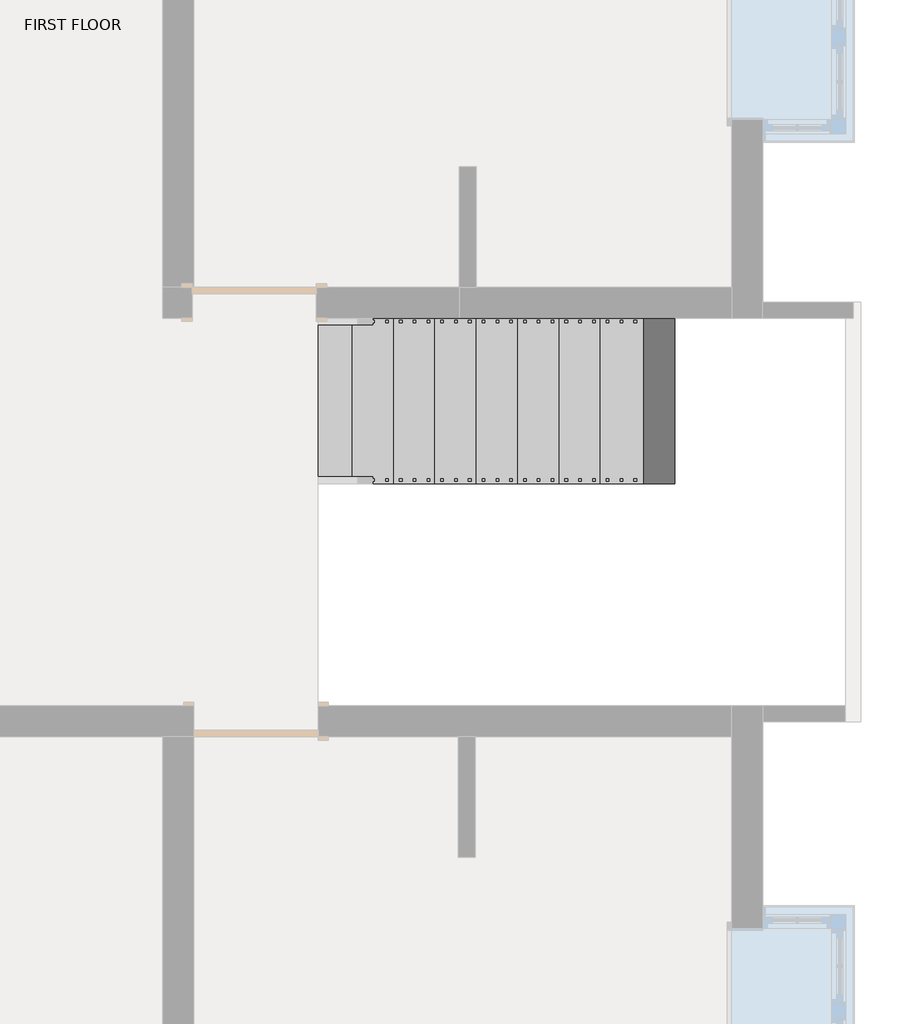
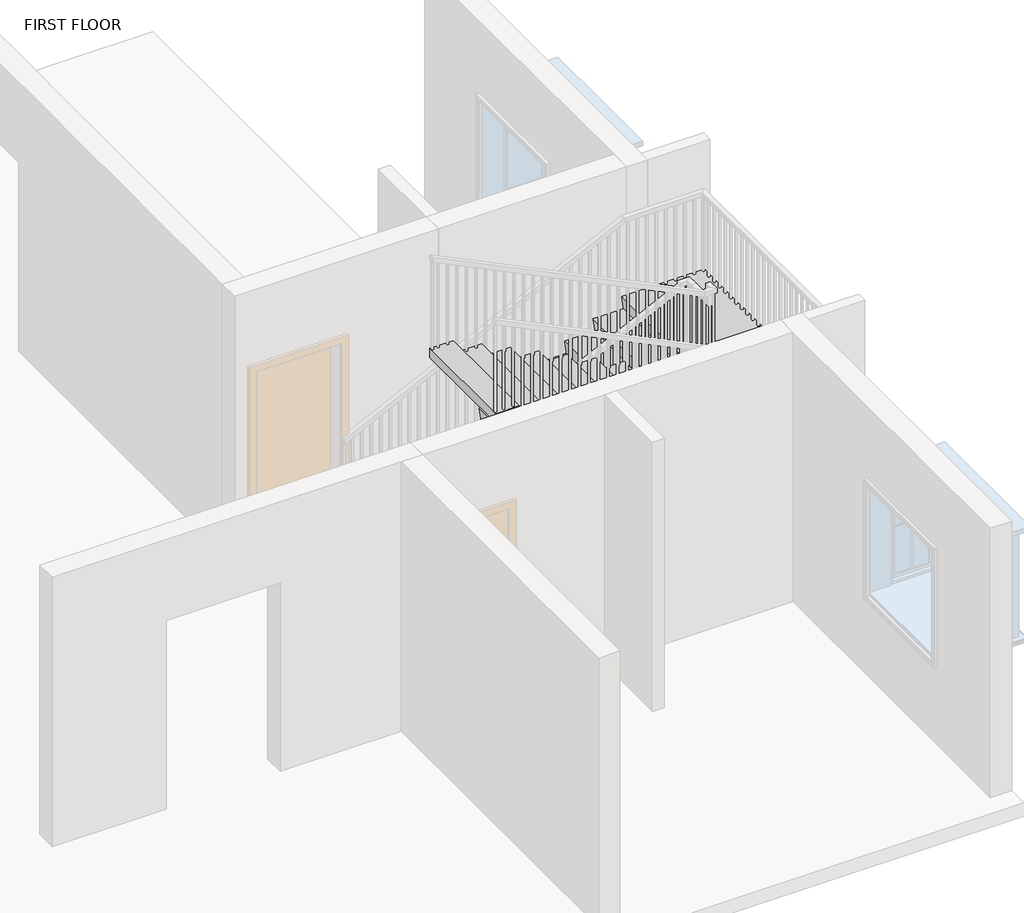
# One storey, part 3 of 6: 1 railing, 1 stair flight.
"""IFC4 building model written with IfcOpenShell, lengths in millimetres."""

from ifc_helpers import new_model, si_unit, frame, origin, place, context, project, spatial, polyline, outline, extrude, faceted_brep, element, save

model = new_model("IFC4")

# Units and contexts
model_context = context("Model", 3, world=origin())
ifc_project = project(units=[si_unit("LENGTHUNIT", "METRE", prefix="MILLI")], contexts=[model_context])

# Site, building, storey
site = spatial("IfcSite", under=ifc_project)
building = spatial("IfcBuilding", under=site)
storey = spatial("IfcBuildingStorey", under=building, Name="FIRST FLOOR", Elevation=3200.4)

# Railing
placement = place(None, origin())
element("IfcRailing", 1, ObjectType="Handrail - Rectangular", at=placement, inside=storey, context=model_context, shape_type="SolidModel", body=[
    faceted_brep([(3126.2584916, -947.666654, 4260.2727273), (3126.2584916, -947.666654, 4203.7956113), (3126.2584916, -998.466654, 4203.7956113), (3126.2584916, -998.466654, 4260.2727273), (6044.5829507, -947.666654, 5677.9823634), (6095.3829507, -947.666654, 5646.1836718), (6095.3829507, -998.466654, 5646.1836718), (6044.5829507, -998.466654, 5677.9823634), (6044.5829507, -947.666654, 5715.0), (6095.3829507, -947.666654, 5664.2), (6095.3829507, -998.466654, 5664.2), (6044.5829507, -998.466654, 5715.0), (6171.5829507, -947.666654, 5715.0), (6171.5829507, -947.666654, 5664.2), (6120.7829507, -998.466654, 5664.2), (6120.7829507, -998.466654, 5715.0), (6171.5829507, -1074.666654, 5715.0), (6171.5829507, -1074.666654, 5664.2), (6120.7829507, -1074.666654, 5664.2), (6120.7829507, -1074.666654, 5715.0), (6171.5829507, -1341.366654, 5715.0), (6171.5829507, -1392.166654, 5664.2), (6120.7829507, -1392.166654, 5664.2), (6120.7829507, -1341.366654, 5715.0), (6171.5829507, -1341.366654, 5897.4903639), (6171.5829507, -1392.166654, 5846.6903639), (6120.7829507, -1392.166654, 5846.6903639), (6120.7829507, -1341.366654, 5897.4903639), (6171.5829507, -1468.366654, 5897.4903639), (6171.5829507, -1468.366654, 5846.6903639), (6120.7829507, -1417.566654, 5846.6903639), (6120.7829507, -1417.566654, 5897.4903639), (6044.5829507, -1468.366654, 5897.4903639), (6032.8967309, -1468.366654, 5846.6903639), (6032.8967309, -1417.566654, 5846.6903639), (6044.5829507, -1417.566654, 5897.4903639), (3126.2584916, -1468.366654, 7315.2), (3126.2584916, -1417.566654, 7315.2), (3126.2584916, -1417.566654, 7258.722884), (3126.2584916, -1468.366654, 7258.722884)], [[[0, 1, 2, 3]], [[1, 0, 4, 5]], [[2, 1, 5, 6]], [[3, 2, 6, 7]], [[0, 3, 7, 4]], [[5, 4, 8, 9]], [[6, 5, 9, 10]], [[7, 6, 10, 11]], [[4, 7, 11, 8]], [[9, 8, 12, 13]], [[10, 9, 13, 14]], [[11, 10, 14, 15]], [[8, 11, 15, 12]], [[13, 12, 16, 17]], [[14, 13, 17, 18]], [[15, 14, 18, 19]], [[12, 15, 19, 16]], [[17, 16, 20, 21]], [[18, 17, 21, 22]], [[19, 18, 22, 23]], [[16, 19, 23, 20]], [[21, 20, 24, 25]], [[22, 21, 25, 26]], [[23, 22, 26, 27]], [[20, 23, 27, 24]], [[25, 24, 28, 29]], [[26, 25, 29, 30]], [[27, 26, 30, 31]], [[24, 27, 31, 28]], [[29, 28, 32, 33]], [[30, 29, 33, 34]], [[31, 30, 34, 35]], [[28, 31, 35, 32]], [[36, 37, 38, 39]], [[33, 32, 36, 39]], [[34, 33, 39, 38]], [[35, 34, 38, 37]], [[32, 35, 37, 36]]]),
    extrude(outline(polyline([(7218.3778093, 3209.3079507), (7227.6322184, 3190.2579507), (6255.3272727, 3190.2579507), (6255.3272727, 3209.3079507), (7218.3778093, 3209.3079507)])), frame((0.0, -1452.491654, 0.0), z_axis=(0.0, 1.0, 0.0), x_axis=(0.0, 0.0, 1.0)), (0.0, 0.0, 1.0), 19.05),
    extrude(outline(polyline([(7169.0209605, 3310.9079507), (7178.2753696, 3291.8579507), (6255.3272727, 3291.8579507), (6255.3272727, 3310.9079507), (7169.0209605, 3310.9079507)])), frame((0.0, -1452.491654, 0.0), z_axis=(0.0, 1.0, 0.0), x_axis=(0.0, 0.0, 1.0)), (0.0, 0.0, 1.0), 19.05),
    extrude(outline(polyline([(7119.6641117, 3412.5079507), (7128.9185208, 3393.4579507), (6109.8545455, 3393.4579507), (6109.8545455, 3412.5079507), (7119.6641117, 3412.5079507)])), frame((0.0, -1452.491654, 0.0), z_axis=(0.0, 1.0, 0.0), x_axis=(0.0, 0.0, 1.0)), (0.0, 0.0, 1.0), 19.05),
    extrude(outline(polyline([(7070.3072629, 3514.1079507), (7079.5616721, 3495.0579507), (6109.8545455, 3495.0579507), (6109.8545455, 3514.1079507), (7070.3072629, 3514.1079507)])), frame((0.0, -1452.491654, 0.0), z_axis=(0.0, 1.0, 0.0), x_axis=(0.0, 0.0, 1.0)), (0.0, 0.0, 1.0), 19.05),
    extrude(outline(polyline([(7020.9504141, 3615.7079507), (7030.2048233, 3596.6579507), (6109.8545455, 3596.6579507), (6109.8545455, 3615.7079507), (7020.9504141, 3615.7079507)])), frame((0.0, -1452.491654, 0.0), z_axis=(0.0, 1.0, 0.0), x_axis=(0.0, 0.0, 1.0)), (0.0, 0.0, 1.0), 19.05),
    extrude(outline(polyline([(6971.5935653, 3717.3079507), (6980.8479745, 3698.2579507), (5964.3818182, 3698.2579507), (5964.3818182, 3717.3079507), (6971.5935653, 3717.3079507)])), frame((0.0, -1452.491654, 0.0), z_axis=(0.0, 1.0, 0.0), x_axis=(0.0, 0.0, 1.0)), (0.0, 0.0, 1.0), 19.05),
    extrude(outline(polyline([(6922.2367166, 3818.9079507), (6931.4911257, 3799.8579507), (5964.3818182, 3799.8579507), (5964.3818182, 3818.9079507), (6922.2367166, 3818.9079507)])), frame((0.0, -1452.491654, 0.0), z_axis=(0.0, 1.0, 0.0), x_axis=(0.0, 0.0, 1.0)), (0.0, 0.0, 1.0), 19.05),
    extrude(outline(polyline([(6872.8798678, 3920.5079507), (6882.1342769, 3901.4579507), (5964.3818182, 3901.4579507), (5964.3818182, 3920.5079507), (6872.8798678, 3920.5079507)])), frame((0.0, -1452.491654, 0.0), z_axis=(0.0, 1.0, 0.0), x_axis=(0.0, 0.0, 1.0)), (0.0, 0.0, 1.0), 19.05),
    extrude(outline(polyline([(6823.523019, 4022.1079507), (6832.7774281, 4003.0579507), (5818.9090909, 4003.0579507), (5818.9090909, 4022.1079507), (6823.523019, 4022.1079507)])), frame((0.0, -1452.491654, 0.0), z_axis=(0.0, 1.0, 0.0), x_axis=(0.0, 0.0, 1.0)), (0.0, 0.0, 1.0), 19.05),
    extrude(outline(polyline([(6774.1661702, 4123.7079507), (6783.4205793, 4104.6579507), (5818.9090909, 4104.6579507), (5818.9090909, 4123.7079507), (6774.1661702, 4123.7079507)])), frame((0.0, -1452.491654, 0.0), z_axis=(0.0, 1.0, 0.0), x_axis=(0.0, 0.0, 1.0)), (0.0, 0.0, 1.0), 19.05),
    extrude(outline(polyline([(6724.8093214, 4225.3079507), (6734.0637306, 4206.2579507), (5818.9090909, 4206.2579507), (5818.9090909, 4225.3079507), (6724.8093214, 4225.3079507)])), frame((0.0, -1452.491654, 0.0), z_axis=(0.0, 1.0, 0.0), x_axis=(0.0, 0.0, 1.0)), (0.0, 0.0, 1.0), 19.05),
    extrude(outline(polyline([(6675.4524726, 4326.9079507), (6684.7068818, 4307.8579507), (5673.4363636, 4307.8579507), (5673.4363636, 4326.9079507), (6675.4524726, 4326.9079507)])), frame((0.0, -1452.491654, 0.0), z_axis=(0.0, 1.0, 0.0), x_axis=(0.0, 0.0, 1.0)), (0.0, 0.0, 1.0), 19.05),
    extrude(outline(polyline([(6626.0956238, 4428.5079507), (6635.350033, 4409.4579507), (5673.4363636, 4409.4579507), (5673.4363636, 4428.5079507), (6626.0956238, 4428.5079507)])), frame((0.0, -1452.491654, 0.0), z_axis=(0.0, 1.0, 0.0), x_axis=(0.0, 0.0, 1.0)), (0.0, 0.0, 1.0), 19.05),
    extrude(outline(polyline([(6576.7387751, 4530.1079507), (6585.9931842, 4511.0579507), (5673.4363636, 4511.0579507), (5673.4363636, 4530.1079507), (6576.7387751, 4530.1079507)])), frame((0.0, -1452.491654, 0.0), z_axis=(0.0, 1.0, 0.0), x_axis=(0.0, 0.0, 1.0)), (0.0, 0.0, 1.0), 19.05),
    extrude(outline(polyline([(6527.3819263, 4631.7079507), (6536.6363354, 4612.6579507), (5527.9636364, 4612.6579507), (5527.9636364, 4631.7079507), (6527.3819263, 4631.7079507)])), frame((0.0, -1452.491654, 0.0), z_axis=(0.0, 1.0, 0.0), x_axis=(0.0, 0.0, 1.0)), (0.0, 0.0, 1.0), 19.05),
    extrude(outline(polyline([(6478.0250775, 4733.3079507), (6487.2794866, 4714.2579507), (5527.9636364, 4714.2579507), (5527.9636364, 4733.3079507), (6478.0250775, 4733.3079507)])), frame((0.0, -1452.491654, 0.0), z_axis=(0.0, 1.0, 0.0), x_axis=(0.0, 0.0, 1.0)), (0.0, 0.0, 1.0), 19.05),
    extrude(outline(polyline([(6428.6682287, 4834.9079507), (6437.9226379, 4815.8579507), (5527.9636364, 4815.8579507), (5527.9636364, 4834.9079507), (6428.6682287, 4834.9079507)])), frame((0.0, -1452.491654, 0.0), z_axis=(0.0, 1.0, 0.0), x_axis=(0.0, 0.0, 1.0)), (0.0, 0.0, 1.0), 19.05),
    extrude(outline(polyline([(6379.3113799, 4936.5079507), (6388.5657891, 4917.4579507), (5382.4909091, 4917.4579507), (5382.4909091, 4936.5079507), (6379.3113799, 4936.5079507)])), frame((0.0, -1452.491654, 0.0), z_axis=(0.0, 1.0, 0.0), x_axis=(0.0, 0.0, 1.0)), (0.0, 0.0, 1.0), 19.05),
    extrude(outline(polyline([(6329.9545311, 5038.1079507), (6339.2089403, 5019.0579507), (5382.4909091, 5019.0579507), (5382.4909091, 5038.1079507), (6329.9545311, 5038.1079507)])), frame((0.0, -1452.491654, 0.0), z_axis=(0.0, 1.0, 0.0), x_axis=(0.0, 0.0, 1.0)), (0.0, 0.0, 1.0), 19.05),
    extrude(outline(polyline([(6280.5976824, 5139.7079507), (6289.8520915, 5120.6579507), (5382.4909091, 5120.6579507), (5382.4909091, 5139.7079507), (6280.5976824, 5139.7079507)])), frame((0.0, -1452.491654, 0.0), z_axis=(0.0, 1.0, 0.0), x_axis=(0.0, 0.0, 1.0)), (0.0, 0.0, 1.0), 19.05),
    extrude(outline(polyline([(6231.159384, 5241.3079507), (6240.4137931, 5222.2579507), (5237.0181818, 5222.2579507), (5237.0181818, 5241.3079507), (6231.159384, 5241.3079507)])), frame((0.0, -1452.491654, 0.0), z_axis=(0.0, 1.0, 0.0), x_axis=(0.0, 0.0, 1.0)), (0.0, 0.0, 1.0), 19.05),
    extrude(outline(polyline([(6181.8839848, 5342.9079507), (6191.1383939, 5323.8579507), (5237.0181818, 5323.8579507), (5237.0181818, 5342.9079507), (6181.8839848, 5342.9079507)])), frame((0.0, -1452.491654, 0.0), z_axis=(0.0, 1.0, 0.0), x_axis=(0.0, 0.0, 1.0)), (0.0, 0.0, 1.0), 19.05),
    extrude(outline(polyline([(6132.527136, 5444.5079507), (6141.7815452, 5425.4579507), (5237.0181818, 5425.4579507), (5237.0181818, 5444.5079507), (6132.527136, 5444.5079507)])), frame((0.0, -1452.491654, 0.0), z_axis=(0.0, 1.0, 0.0), x_axis=(0.0, 0.0, 1.0)), (0.0, 0.0, 1.0), 19.05),
    extrude(outline(polyline([(6083.1702872, 5546.1079507), (6092.4246964, 5527.0579507), (5091.5454545, 5527.0579507), (5091.5454545, 5546.1079507), (6083.1702872, 5546.1079507)])), frame((0.0, -1452.491654, 0.0), z_axis=(0.0, 1.0, 0.0), x_axis=(0.0, 0.0, 1.0)), (0.0, 0.0, 1.0), 19.05),
    extrude(outline(polyline([(6033.8134384, 5647.7079507), (6043.0678476, 5628.6579507), (5091.5454545, 5628.6579507), (5091.5454545, 5647.7079507), (6033.8134384, 5647.7079507)])), frame((0.0, -1452.491654, 0.0), z_axis=(0.0, 1.0, 0.0), x_axis=(0.0, 0.0, 1.0)), (0.0, 0.0, 1.0), 19.05),
    extrude(outline(polyline([(5984.4565897, 5749.3079507), (5993.7109988, 5730.2579507), (5091.5454545, 5730.2579507), (5091.5454545, 5749.3079507), (5984.4565897, 5749.3079507)])), frame((0.0, -1452.491654, 0.0), z_axis=(0.0, 1.0, 0.0), x_axis=(0.0, 0.0, 1.0)), (0.0, 0.0, 1.0), 19.05),
    extrude(outline(polyline([(5935.0997409, 5850.9079507), (5944.35415, 5831.8579507), (4946.0727273, 5831.8579507), (4946.0727273, 5850.9079507), (5935.0997409, 5850.9079507)])), frame((0.0, -1452.491654, 0.0), z_axis=(0.0, 1.0, 0.0), x_axis=(0.0, 0.0, 1.0)), (0.0, 0.0, 1.0), 19.05),
    extrude(outline(polyline([(5885.7428921, 5952.5079507), (5894.9973012, 5933.4579507), (4946.0727273, 5933.4579507), (4946.0727273, 5952.5079507), (5885.7428921, 5952.5079507)])), frame((0.0, -1452.491654, 0.0), z_axis=(0.0, 1.0, 0.0), x_axis=(0.0, 0.0, 1.0)), (0.0, 0.0, 1.0), 19.05),
    extrude(outline(polyline([(5836.3860433, 6054.1079507), (5845.6404524, 6035.0579507), (4946.0727273, 6035.0579507), (4946.0727273, 6054.1079507), (5836.3860433, 6054.1079507)])), frame((0.0, -1452.491654, 0.0), z_axis=(0.0, 1.0, 0.0), x_axis=(0.0, 0.0, 1.0)), (0.0, 0.0, 1.0), 19.05),
    extrude(outline(polyline([(6136.6579507, -1369.941654), (6155.7079507, -1369.941654), (6155.7079507, -1388.991654), (6136.6579507, -1388.991654), (6136.6579507, -1369.941654)])), frame((0.0, 0.0, 4800.6), z_axis=(0.0, 0.0, 1.0), x_axis=(1.0, 0.0, 0.0)), (0.0, 0.0, 1.0), 1046.0903639),
    extrude(outline(polyline([(6136.6579507, -1268.341654), (6155.7079507, -1268.341654), (6155.7079507, -1287.391654), (6136.6579507, -1287.391654), (6136.6579507, -1268.341654)])), frame((0.0, 0.0, 4800.6), z_axis=(0.0, 0.0, 1.0), x_axis=(1.0, 0.0, 0.0)), (0.0, 0.0, 1.0), 863.6),
    extrude(outline(polyline([(6136.6579507, -1166.741654), (6155.7079507, -1166.741654), (6155.7079507, -1185.791654), (6136.6579507, -1185.791654), (6136.6579507, -1166.741654)])), frame((0.0, 0.0, 4800.6), z_axis=(0.0, 0.0, 1.0), x_axis=(1.0, 0.0, 0.0)), (0.0, 0.0, 1.0), 863.6),
    extrude(outline(polyline([(6136.6579507, -1065.141654), (6155.7079507, -1065.141654), (6155.7079507, -1084.191654), (6136.6579507, -1084.191654), (6136.6579507, -1065.141654)])), frame((0.0, 0.0, 4800.6), z_axis=(0.0, 0.0, 1.0), x_axis=(1.0, 0.0, 0.0)), (0.0, 0.0, 1.0), 863.6),
    extrude(outline(polyline([(6063.1334916, -982.591654), (6063.1334916, -963.541654), (6082.1834916, -963.541654), (6082.1834916, -982.591654), (6063.1334916, -982.591654)])), frame((0.0, 0.0, 4655.1272727), z_axis=(0.0, 0.0, 1.0), x_axis=(1.0, 0.0, 0.0)), (0.0, 0.0, 1.0), 1009.0727273),
    extrude(outline(polyline([(5590.4145818, 5980.5834916), (5581.1601727, 5961.5334916), (4655.1272727, 5961.5334916), (4655.1272727, 5980.5834916), (5590.4145818, 5980.5834916)])), frame((0.0, -982.591654, 0.0), z_axis=(0.0, 1.0, 0.0), x_axis=(0.0, 0.0, 1.0)), (0.0, 0.0, 1.0), 19.05),
    extrude(outline(polyline([(5541.057733, 5878.9834916), (5531.8033239, 5859.9334916), (4655.1272727, 5859.9334916), (4655.1272727, 5878.9834916), (5541.057733, 5878.9834916)])), frame((0.0, -982.591654, 0.0), z_axis=(0.0, 1.0, 0.0), x_axis=(0.0, 0.0, 1.0)), (0.0, 0.0, 1.0), 19.05),
    extrude(outline(polyline([(5491.7008843, 5777.3834916), (5482.4464751, 5758.3334916), (4509.6545455, 5758.3334916), (4509.6545455, 5777.3834916), (5491.7008843, 5777.3834916)])), frame((0.0, -982.591654, 0.0), z_axis=(0.0, 1.0, 0.0), x_axis=(0.0, 0.0, 1.0)), (0.0, 0.0, 1.0), 19.05),
    extrude(outline(polyline([(5442.3440355, 5675.7834916), (5433.0896263, 5656.7334916), (4509.6545455, 5656.7334916), (4509.6545455, 5675.7834916), (5442.3440355, 5675.7834916)])), frame((0.0, -982.591654, 0.0), z_axis=(0.0, 1.0, 0.0), x_axis=(0.0, 0.0, 1.0)), (0.0, 0.0, 1.0), 19.05),
    extrude(outline(polyline([(5392.9871867, 5574.1834916), (5383.7327775, 5555.1334916), (4509.6545455, 5555.1334916), (4509.6545455, 5574.1834916), (5392.9871867, 5574.1834916)])), frame((0.0, -982.591654, 0.0), z_axis=(0.0, 1.0, 0.0), x_axis=(0.0, 0.0, 1.0)), (0.0, 0.0, 1.0), 19.05),
    extrude(outline(polyline([(5343.6303379, 5472.5834916), (5334.3759288, 5453.5334916), (4364.1818182, 5453.5334916), (4364.1818182, 5472.5834916), (5343.6303379, 5472.5834916)])), frame((0.0, -982.591654, 0.0), z_axis=(0.0, 1.0, 0.0), x_axis=(0.0, 0.0, 1.0)), (0.0, 0.0, 1.0), 19.05),
    extrude(outline(polyline([(5294.2734891, 5370.9834916), (5285.01908, 5351.9334916), (4364.1818182, 5351.9334916), (4364.1818182, 5370.9834916), (5294.2734891, 5370.9834916)])), frame((0.0, -982.591654, 0.0), z_axis=(0.0, 1.0, 0.0), x_axis=(0.0, 0.0, 1.0)), (0.0, 0.0, 1.0), 19.05),
    extrude(outline(polyline([(5244.9166403, 5269.3834916), (5235.6622312, 5250.3334916), (4364.1818182, 5250.3334916), (4364.1818182, 5269.3834916), (5244.9166403, 5269.3834916)])), frame((0.0, -982.591654, 0.0), z_axis=(0.0, 1.0, 0.0), x_axis=(0.0, 0.0, 1.0)), (0.0, 0.0, 1.0), 19.05),
    extrude(outline(polyline([(5195.5597915, 5167.7834916), (5186.3053824, 5148.7334916), (4218.7090909, 5148.7334916), (4218.7090909, 5167.7834916), (5195.5597915, 5167.7834916)])), frame((0.0, -982.591654, 0.0), z_axis=(0.0, 1.0, 0.0), x_axis=(0.0, 0.0, 1.0)), (0.0, 0.0, 1.0), 19.05),
    extrude(outline(polyline([(5146.2029428, 5066.1834916), (5136.9485336, 5047.1334916), (4218.7090909, 5047.1334916), (4218.7090909, 5066.1834916), (5146.2029428, 5066.1834916)])), frame((0.0, -982.591654, 0.0), z_axis=(0.0, 1.0, 0.0), x_axis=(0.0, 0.0, 1.0)), (0.0, 0.0, 1.0), 19.05),
    extrude(outline(polyline([(5096.846094, 4964.5834916), (5087.5916848, 4945.5334916), (4218.7090909, 4945.5334916), (4218.7090909, 4964.5834916), (5096.846094, 4964.5834916)])), frame((0.0, -982.591654, 0.0), z_axis=(0.0, 1.0, 0.0), x_axis=(0.0, 0.0, 1.0)), (0.0, 0.0, 1.0), 19.05),
    extrude(outline(polyline([(5047.4892452, 4862.9834916), (5038.234836, 4843.9334916), (4073.2363636, 4843.9334916), (4073.2363636, 4862.9834916), (5047.4892452, 4862.9834916)])), frame((0.0, -982.591654, 0.0), z_axis=(0.0, 1.0, 0.0), x_axis=(0.0, 0.0, 1.0)), (0.0, 0.0, 1.0), 19.05),
    extrude(outline(polyline([(4998.1323964, 4761.3834916), (4988.8779873, 4742.3334916), (4073.2363636, 4742.3334916), (4073.2363636, 4761.3834916), (4998.1323964, 4761.3834916)])), frame((0.0, -982.591654, 0.0), z_axis=(0.0, 1.0, 0.0), x_axis=(0.0, 0.0, 1.0)), (0.0, 0.0, 1.0), 19.05),
    extrude(outline(polyline([(4948.7755476, 4659.7834916), (4939.5211385, 4640.7334916), (4073.2363636, 4640.7334916), (4073.2363636, 4659.7834916), (4948.7755476, 4659.7834916)])), frame((0.0, -982.591654, 0.0), z_axis=(0.0, 1.0, 0.0), x_axis=(0.0, 0.0, 1.0)), (0.0, 0.0, 1.0), 19.05),
    extrude(outline(polyline([(4899.4186988, 4558.1834916), (4890.1642897, 4539.1334916), (3927.7636364, 4539.1334916), (3927.7636364, 4558.1834916), (4899.4186988, 4558.1834916)])), frame((0.0, -982.591654, 0.0), z_axis=(0.0, 1.0, 0.0), x_axis=(0.0, 0.0, 1.0)), (0.0, 0.0, 1.0), 19.05),
    extrude(outline(polyline([(4850.0618501, 4456.5834916), (4840.8074409, 4437.5334916), (3927.7636364, 4437.5334916), (3927.7636364, 4456.5834916), (4850.0618501, 4456.5834916)])), frame((0.0, -982.591654, 0.0), z_axis=(0.0, 1.0, 0.0), x_axis=(0.0, 0.0, 1.0)), (0.0, 0.0, 1.0), 19.05),
    extrude(outline(polyline([(4800.7050013, 4354.9834916), (4791.4505921, 4335.9334916), (3927.7636364, 4335.9334916), (3927.7636364, 4354.9834916), (4800.7050013, 4354.9834916)])), frame((0.0, -982.591654, 0.0), z_axis=(0.0, 1.0, 0.0), x_axis=(0.0, 0.0, 1.0)), (0.0, 0.0, 1.0), 19.05),
    extrude(outline(polyline([(4751.3481525, 4253.3834916), (4742.0937433, 4234.3334916), (3782.2909091, 4234.3334916), (3782.2909091, 4253.3834916), (4751.3481525, 4253.3834916)])), frame((0.0, -982.591654, 0.0), z_axis=(0.0, 1.0, 0.0), x_axis=(0.0, 0.0, 1.0)), (0.0, 0.0, 1.0), 19.05),
    extrude(outline(polyline([(4701.9913037, 4151.7834916), (4692.7368946, 4132.7334916), (3782.2909091, 4132.7334916), (3782.2909091, 4151.7834916), (4701.9913037, 4151.7834916)])), frame((0.0, -982.591654, 0.0), z_axis=(0.0, 1.0, 0.0), x_axis=(0.0, 0.0, 1.0)), (0.0, 0.0, 1.0), 19.05),
    extrude(outline(polyline([(4652.6344549, 4050.1834916), (4643.3800458, 4031.1334916), (3782.2909091, 4031.1334916), (3782.2909091, 4050.1834916), (4652.6344549, 4050.1834916)])), frame((0.0, -982.591654, 0.0), z_axis=(0.0, 1.0, 0.0), x_axis=(0.0, 0.0, 1.0)), (0.0, 0.0, 1.0), 19.05),
    extrude(outline(polyline([(4603.2776061, 3948.5834916), (4594.023197, 3929.5334916), (3636.8181818, 3929.5334916), (3636.8181818, 3948.5834916), (4603.2776061, 3948.5834916)])), frame((0.0, -982.591654, 0.0), z_axis=(0.0, 1.0, 0.0), x_axis=(0.0, 0.0, 1.0)), (0.0, 0.0, 1.0), 19.05),
    extrude(outline(polyline([(4553.9207573, 3846.9834916), (4544.6663482, 3827.9334916), (3636.8181818, 3827.9334916), (3636.8181818, 3846.9834916), (4553.9207573, 3846.9834916)])), frame((0.0, -982.591654, 0.0), z_axis=(0.0, 1.0, 0.0), x_axis=(0.0, 0.0, 1.0)), (0.0, 0.0, 1.0), 19.05),
    extrude(outline(polyline([(4504.5639086, 3745.3834916), (4495.3094994, 3726.3334916), (3636.8181818, 3726.3334916), (3636.8181818, 3745.3834916), (4504.5639086, 3745.3834916)])), frame((0.0, -982.591654, 0.0), z_axis=(0.0, 1.0, 0.0), x_axis=(0.0, 0.0, 1.0)), (0.0, 0.0, 1.0), 19.05),
    extrude(outline(polyline([(4455.2070598, 3643.7834916), (4445.9526506, 3624.7334916), (3491.3454545, 3624.7334916), (3491.3454545, 3643.7834916), (4455.2070598, 3643.7834916)])), frame((0.0, -982.591654, 0.0), z_axis=(0.0, 1.0, 0.0), x_axis=(0.0, 0.0, 1.0)), (0.0, 0.0, 1.0), 19.05),
    extrude(outline(polyline([(4405.850211, 3542.1834916), (4396.5958018, 3523.1334916), (3491.3454545, 3523.1334916), (3491.3454545, 3542.1834916), (4405.850211, 3542.1834916)])), frame((0.0, -982.591654, 0.0), z_axis=(0.0, 1.0, 0.0), x_axis=(0.0, 0.0, 1.0)), (0.0, 0.0, 1.0), 19.05),
    extrude(outline(polyline([(4356.4933622, 3440.5834916), (4347.2389531, 3421.5334916), (3491.3454545, 3421.5334916), (3491.3454545, 3440.5834916), (4356.4933622, 3440.5834916)])), frame((0.0, -982.591654, 0.0), z_axis=(0.0, 1.0, 0.0), x_axis=(0.0, 0.0, 1.0)), (0.0, 0.0, 1.0), 19.05),
    extrude(outline(polyline([(4307.1365134, 3338.9834916), (4297.8821043, 3319.9334916), (3345.8727273, 3319.9334916), (3345.8727273, 3338.9834916), (4307.1365134, 3338.9834916)])), frame((0.0, -982.591654, 0.0), z_axis=(0.0, 1.0, 0.0), x_axis=(0.0, 0.0, 1.0)), (0.0, 0.0, 1.0), 19.05),
    extrude(outline(polyline([(4257.7796646, 3237.3834916), (4248.5252555, 3218.3334916), (3345.8727273, 3218.3334916), (3345.8727273, 3237.3834916), (4257.7796646, 3237.3834916)])), frame((0.0, -982.591654, 0.0), z_axis=(0.0, 1.0, 0.0), x_axis=(0.0, 0.0, 1.0)), (0.0, 0.0, 1.0), 19.05),
    extrude(outline(polyline([(6136.6579507, -1433.441654), (6155.7079507, -1433.441654), (6155.7079507, -1452.491654), (6136.6579507, -1452.491654), (6136.6579507, -1433.441654)])), frame((0.0, 0.0, 4800.6), z_axis=(0.0, 0.0, 1.0), x_axis=(1.0, 0.0, 0.0)), (0.0, 0.0, 1.0), 1046.0903639),
    extrude(outline(polyline([(6136.6579507, -982.591654), (6136.6579507, -963.541654), (6155.7079507, -963.541654), (6155.7079507, -982.591654), (6136.6579507, -982.591654)])), frame((0.0, 0.0, 4800.6), z_axis=(0.0, 0.0, 1.0), x_axis=(1.0, 0.0, 0.0)), (0.0, 0.0, 1.0), 863.6),
    extrude(outline(polyline([(7249.4684749, 3145.3084916), (7258.722884, 3126.2584916), (6255.3272727, 3126.2584916), (6255.3272727, 3145.3084916), (7249.4684749, 3145.3084916)])), frame((0.0, -1452.491654, 0.0), z_axis=(0.0, 1.0, 0.0), x_axis=(0.0, 0.0, 1.0)), (0.0, 0.0, 1.0), 19.05),
    extrude(outline(polyline([(4213.0500204, 3145.3084916), (4203.7956113, 3126.2584916), (3345.8727273, 3126.2584916), (3345.8727273, 3145.3084916), (4213.0500204, 3145.3084916)])), frame((0.0, -982.591654, 0.0), z_axis=(0.0, 1.0, 0.0), x_axis=(0.0, 0.0, 1.0)), (0.0, 0.0, 1.0), 19.05),
])

# Stair flight
element("IfcStairFlight", 2, ObjectType="3/4\" Nosing", at=placement, inside=storey, context=model_context, shape_type="Brep", body=[
    faceted_brep([(3126.2584916, 220.733346, 3345.8727273), (3126.2584916, -998.466654, 3345.8727273), (3396.6329507, -998.466654, 3345.8727273), (3396.6329507, 220.733346, 3345.8727273), (3396.6329507, 220.733346, 3282.3727273), (3134.5739678, 220.733346, 3282.3727273), (3134.5739678, -998.466654, 3282.3727273), (3396.6329507, -998.466654, 3282.3727273), (3377.5829507, 220.733346, 3491.3454545), (3377.5829507, -998.466654, 3491.3454545), (3411.0096137, -998.466654, 3491.3454545), (3701.4329507, -998.466654, 3491.3454545), (3701.4329507, 220.733346, 3491.3454545), (3411.0096137, 220.733346, 3491.3454545), (3701.4329507, 220.733346, 3420.9838654), (3411.0096137, 220.733346, 3282.3727273), (3411.0096137, -998.466654, 3282.3727273), (3701.4329507, -998.466654, 3420.9838654), (3682.3829507, 220.733346, 3636.8181818), (3682.3829507, -998.466654, 3636.8181818), (4006.2329507, -998.466654, 3636.8181818), (4006.2329507, 220.733346, 3636.8181818), (4006.2329507, 220.733346, 3566.4565927), (4006.2329507, -998.466654, 3566.4565927), (3987.1829507, 220.733346, 3782.2909091), (3987.1829507, -998.466654, 3782.2909091), (4311.0329507, -998.466654, 3782.2909091), (4311.0329507, 220.733346, 3782.2909091), (4311.0329507, 220.733346, 3711.9293199), (4311.0329507, -998.466654, 3711.9293199), (4291.9829507, 220.733346, 3927.7636364), (4291.9829507, -998.466654, 3927.7636364), (4615.8329507, -998.466654, 3927.7636364), (4615.8329507, 220.733346, 3927.7636364), (4615.8329507, 220.733346, 3857.4020472), (4615.8329507, -998.466654, 3857.4020472), (4596.7829507, 220.733346, 4073.2363636), (4596.7829507, -998.466654, 4073.2363636), (4920.6329507, -998.466654, 4073.2363636), (4920.6329507, 220.733346, 4073.2363636), (4920.6329507, 220.733346, 4002.8747745), (4920.6329507, -998.466654, 4002.8747745), (4901.5829507, 220.733346, 4218.7090909), (4901.5829507, -998.466654, 4218.7090909), (5225.4329507, -998.466654, 4218.7090909), (5225.4329507, 220.733346, 4218.7090909), (5225.4329507, 220.733346, 4148.3475018), (5225.4329507, -998.466654, 4148.3475018), (5206.3829507, 220.733346, 4364.1818182), (5206.3829507, -998.466654, 4364.1818182), (5530.2329507, -998.466654, 4364.1818182), (5530.2329507, 220.733346, 4364.1818182), (5530.2329507, 220.733346, 4293.820229), (5530.2329507, -998.466654, 4293.820229), (5511.1829507, 220.733346, 4509.6545455), (5511.1829507, -998.466654, 4509.6545455), (5835.0329507, -998.466654, 4509.6545455), (5835.0329507, 220.733346, 4509.6545455), (5835.0329507, 220.733346, 4439.2929563), (5835.0329507, -998.466654, 4439.2929563), (5815.9829507, 220.733346, 4655.1272727), (5815.9829507, -998.466654, 4655.1272727), (6139.8329507, -998.466654, 4655.1272727), (6139.8329507, 220.733346, 4655.1272727), (6139.8329507, 220.733346, 4584.7656836), (6459.0096137, -998.466654, 4737.1), (6129.0984269, -998.466654, 4737.1), (6101.7329507, -2636.766654, 4800.6), (7009.1350459, -2636.766654, 4800.6), (7009.1350459, 220.733346, 4800.6), (6459.0096137, 220.733346, 4800.6), (6120.7829507, 220.733346, 4800.6), (6120.7829507, -998.466654, 4800.6), (6120.7829507, -1417.566654, 4800.6), (6101.7329507, -1417.566654, 4800.6), (6101.7329507, -2636.766654, 4737.1), (7009.1350459, -2636.766654, 4737.1), (7009.1350459, 220.733346, 4737.1), (6459.0096137, 220.733346, 4737.1), (6120.7829507, -998.466654, 4737.1), (6120.7829507, -1417.566654, 4737.1), (6101.7329507, -1417.566654, 4737.1), (6120.7829507, -2636.766654, 4946.0727273), (6120.7829507, -1417.566654, 4946.0727273), (6087.3562877, -1417.566654, 4946.0727273), (5796.9329507, -1417.566654, 4946.0727273), (5796.9329507, -2636.766654, 4946.0727273), (6087.3562877, -2636.766654, 4946.0727273), (5796.9329507, -2636.766654, 4875.7111381), (6087.3562877, -2636.766654, 4737.1), (6087.3562877, -1417.566654, 4737.1), (5796.9329507, -1417.566654, 4875.7111381), (5815.9829507, -2636.766654, 5091.5454545), (5815.9829507, -1417.566654, 5091.5454545), (5492.1329507, -1417.566654, 5091.5454545), (5492.1329507, -2636.766654, 5091.5454545), (5492.1329507, -2636.766654, 5021.1838654), (5492.1329507, -1417.566654, 5021.1838654), (5511.1829507, -2636.766654, 5237.0181818), (5511.1829507, -1417.566654, 5237.0181818), (5187.3329507, -1417.566654, 5237.0181818), (5187.3329507, -2636.766654, 5237.0181818), (5187.3329507, -2636.766654, 5166.6565927), (5187.3329507, -1417.566654, 5166.6565927), (5206.3829507, -2636.766654, 5382.4909091), (5206.3829507, -1417.566654, 5382.4909091), (4882.5329507, -1417.566654, 5382.4909091), (4882.5329507, -2636.766654, 5382.4909091), (4882.5329507, -2636.766654, 5312.1293199), (4882.5329507, -1417.566654, 5312.1293199), (4901.5829507, -2636.766654, 5527.9636364), (4901.5829507, -1417.566654, 5527.9636364), (4577.7329507, -1417.566654, 5527.9636364), (4577.7329507, -2636.766654, 5527.9636364), (4577.7329507, -2636.766654, 5457.6020472), (4577.7329507, -1417.566654, 5457.6020472), (4596.7829507, -2636.766654, 5673.4363636), (4596.7829507, -1417.566654, 5673.4363636), (4272.9329507, -1417.566654, 5673.4363636), (4272.9329507, -2636.766654, 5673.4363636), (4272.9329507, -2636.766654, 5603.0747745), (4272.9329507, -1417.566654, 5603.0747745), (4291.9829507, -2636.766654, 5818.9090909), (4291.9829507, -1417.566654, 5818.9090909), (3968.1329507, -1417.566654, 5818.9090909), (3968.1329507, -2636.766654, 5818.9090909), (3968.1329507, -2636.766654, 5748.5475018), (3968.1329507, -1417.566654, 5748.5475018), (3987.1829507, -2636.766654, 5964.3818182), (3987.1829507, -1417.566654, 5964.3818182), (3663.3329507, -1417.566654, 5964.3818182), (3663.3329507, -2636.766654, 5964.3818182), (3663.3329507, -2636.766654, 5894.020229), (3663.3329507, -1417.566654, 5894.020229), (3682.3829507, -2636.766654, 6109.8545455), (3682.3829507, -1417.566654, 6109.8545455), (3358.5329507, -1417.566654, 6109.8545455), (3358.5329507, -2636.766654, 6109.8545455), (3358.5329507, -2636.766654, 6039.4929563), (3358.5329507, -1417.566654, 6039.4929563), (3377.5829507, -2636.766654, 6255.3272727), (3377.5829507, -1417.566654, 6255.3272727), (3126.2584916, -1417.566654, 6255.3272727), (3126.2584916, -2636.766654, 6255.3272727), (3126.2584916, -2636.766654, 6150.3512209), (3126.2584916, -1417.566654, 6150.3512209)], [[[0, 1, 2, 3]], [[0, 3, 4, 5]], [[2, 1, 6, 7]], [[8, 9, 10, 11, 12, 13]], [[3, 8, 13, 12, 14, 15, 4]], [[9, 2, 7, 16, 17, 11, 10]], [[18, 19, 20, 21]], [[18, 21, 22, 14, 12]], [[20, 19, 11, 17, 23]], [[24, 25, 26, 27]], [[24, 27, 28, 22, 21]], [[26, 25, 20, 23, 29]], [[30, 31, 32, 33]], [[30, 33, 34, 28, 27]], [[32, 31, 26, 29, 35]], [[36, 37, 38, 39]], [[36, 39, 40, 34, 33]], [[38, 37, 32, 35, 41]], [[42, 43, 44, 45]], [[42, 45, 46, 40, 39]], [[44, 43, 38, 41, 47]], [[48, 49, 50, 51]], [[48, 51, 52, 46, 45]], [[50, 49, 44, 47, 53]], [[54, 55, 56, 57]], [[54, 57, 58, 52, 51]], [[56, 55, 50, 53, 59]], [[60, 61, 62, 63]], [[60, 63, 64, 58, 57]], [[61, 56, 59, 65, 66, 62]], [[67, 68, 69, 70, 71, 72, 73, 74]], [[68, 67, 75, 76]], [[69, 68, 76, 77]], [[63, 71, 70, 69, 77, 78, 64]], [[72, 66, 79]], [[73, 72, 79, 80]], [[74, 73, 80, 81]], [[82, 83, 84, 85, 86, 87]], [[67, 82, 87, 86, 88, 89, 75]], [[83, 74, 81, 90, 91, 85, 84]], [[92, 93, 94, 95]], [[92, 95, 96, 88, 86]], [[94, 93, 85, 91, 97]], [[98, 99, 100, 101]], [[98, 101, 102, 96, 95]], [[100, 99, 94, 97, 103]], [[104, 105, 106, 107]], [[104, 107, 108, 102, 101]], [[106, 105, 100, 103, 109]], [[110, 111, 112, 113]], [[110, 113, 114, 108, 107]], [[112, 111, 106, 109, 115]], [[116, 117, 118, 119]], [[116, 119, 120, 114, 113]], [[118, 117, 112, 115, 121]], [[122, 123, 124, 125]], [[122, 125, 126, 120, 119]], [[124, 123, 118, 121, 127]], [[128, 129, 130, 131]], [[128, 131, 132, 126, 125]], [[130, 129, 124, 127, 133]], [[134, 135, 136, 137]], [[134, 137, 138, 132, 131]], [[136, 135, 130, 133, 139]], [[140, 141, 142, 143]], [[140, 143, 144, 138, 137]], [[142, 141, 136, 139, 145]], [[143, 142, 145, 144]], [[1, 0, 5, 6]], [[3, 2, 9, 8]], [[12, 11, 19, 18]], [[21, 20, 25, 24]], [[27, 26, 31, 30]], [[33, 32, 37, 36]], [[39, 38, 43, 42]], [[45, 44, 49, 48]], [[51, 50, 55, 54]], [[57, 56, 61, 60]], [[63, 62, 66, 72, 71]], [[67, 74, 83, 82]], [[86, 85, 93, 92]], [[95, 94, 99, 98]], [[101, 100, 105, 104]], [[107, 106, 111, 110]], [[113, 112, 117, 116]], [[119, 118, 123, 122]], [[125, 124, 129, 128]], [[131, 130, 135, 134]], [[137, 136, 141, 140]], [[15, 16, 7, 6, 5, 4]], [[16, 15, 14, 22, 28, 34, 40, 46, 52, 58, 64, 78, 65, 59, 53, 47, 41, 35, 29, 23, 17]], [[65, 78, 77, 76, 75, 89, 90, 81, 80, 79, 66]], [[90, 89, 88, 96, 102, 108, 114, 120, 126, 132, 138, 144, 145, 139, 133, 127, 121, 115, 109, 103, 97, 91]]]),
])

save(model, "model.ifc")

# Revit data of these elements
# Type "Handrail - Rectangular"
#   Assembly Code = "C2010400"
#   built-in parameter 1008612 = 0.0416667 (stored number, unit not read)
#   built-in parameter 1008611 = 0.0416667 (stored number, unit not read)
#   built-in parameter 1008609 = 0.333333 (stored number, unit not read)
#   built-in parameter 1008604 = 0.166667 (stored number, unit not read)
#   built-in parameter 1008603 = 0.166667 (stored number, unit not read)
#   Railing Height = 3' - 0"
#   built-in parameter 1008630 = 2
#   built-in parameter 1008610 = 2
#   built-in parameter 1008618 = Baluster - Square : 3/4"
# Element 1 (IfcRailing, "Handrail - Rectangular")
#   Phase Created = New Construction
# Element 2 (IfcStairFlight, "3/4\" Nosing")
#   Phase Created = New Construction
#   Materials on its faces: "Concrete, Cast-in-Place gray"
# Materials
#   "Concrete, Cast-in-Place gray": class "Concrete", colour RGB 192 192 192, transparency 0, Description = "Cast-in-place concrete", Cost = 0
